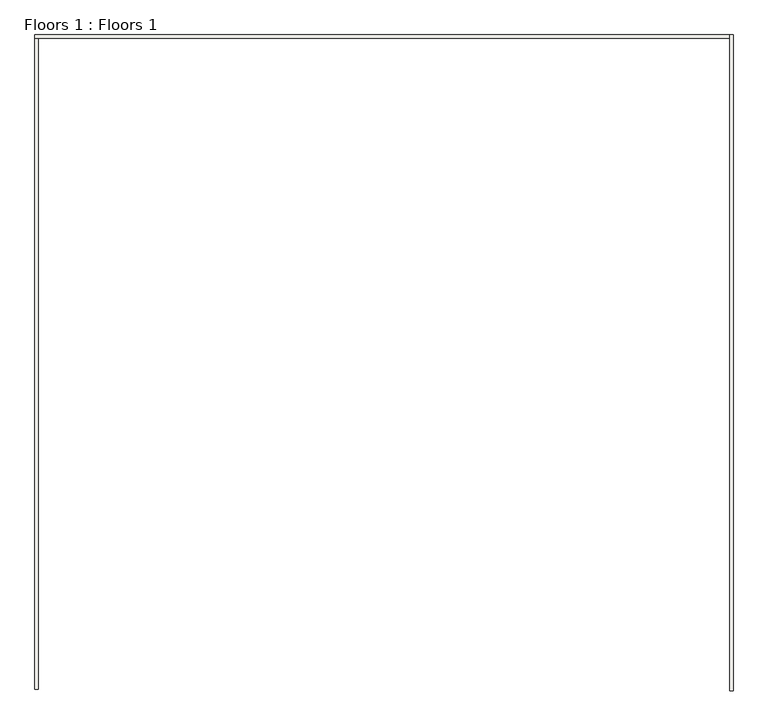
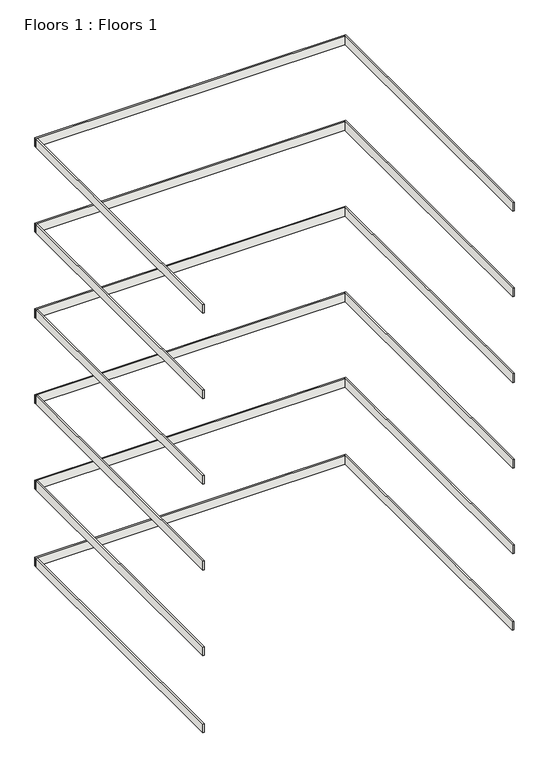
"""IFC4 building model written with IfcOpenShell, lengths in millimetres: slab geometry, Floors 1 : Floors 1."""

from ifc_helpers import new_model, si_unit, frame, origin, origin_with_axes, place, context, project, spatial, polyline, outline, extrude, source, transform, mapped, element, save


def floors_1_floors_1_bc35289f(model_context):
    return source(origin(), model_context, "Body", "SweptSolid", [
        extrude(outline(polyline([(3889.1430349, 10255.9055142), (3889.1430349, 426.1055142), (3838.3430349, 426.1055142), (3838.3430349, 10255.9055142), (3889.1430349, 10255.9055142)])), frame((0.0, 0.0, 14936.2060177), z_axis=(0.0, 0.0, 1.0), x_axis=(1.0, 0.0, 0.0)), (0.0, 0.0, 1.0), 303.7939823),
        extrude(outline(polyline([(3889.1430349, 10255.9055142), (3889.1430349, 426.1055142), (3838.3430349, 426.1055142), (3838.3430349, 10255.9055142), (3889.1430349, 10255.9055142)])), frame((0.0, 0.0, 11887.2), z_axis=(0.0, 0.0, 1.0), x_axis=(1.0, 0.0, 0.0)), (0.0, 0.0, 1.0), 304.8),
        extrude(outline(polyline([(3889.1430349, 10255.9055142), (3889.1430349, 426.1055142), (3838.3430349, 426.1055142), (3838.3430349, 10255.9055142), (3889.1430349, 10255.9055142)])), frame((0.0, 0.0, 8839.6684815), z_axis=(0.0, 0.0, 1.0), x_axis=(1.0, 0.0, 0.0)), (0.0, 0.0, 1.0), 304.3315185),
        extrude(outline(polyline([(3889.1430349, 10255.9055142), (3889.1430349, 426.1055142), (3838.3430349, 426.1055142), (3838.3430349, 10255.9055142), (3889.1430349, 10255.9055142)])), frame((0.0, 0.0, 5791.2), z_axis=(0.0, 0.0, 1.0), x_axis=(1.0, 0.0, 0.0)), (0.0, 0.0, 1.0), 304.8),
        extrude(outline(polyline([(3889.1430349, 10255.9055142), (3889.1430349, 426.1055142), (3838.3430349, 426.1055142), (3838.3430349, 10255.9055142), (3889.1430349, 10255.9055142)])), frame((0.0, 0.0, 2743.2), z_axis=(0.0, 0.0, 1.0), x_axis=(1.0, 0.0, 0.0)), (0.0, 0.0, 1.0), 304.8),
        extrude(outline(polyline([(3889.1430349, 10255.9055142), (3889.1430349, 451.5055142), (3838.3430349, 451.5055142), (3838.3430349, 10255.9055142), (3889.1430349, 10255.9055142)])), origin_with_axes(), (0.0, 0.0, 1.0), 304.8),
        extrude(outline(polyline([(-6575.6569651, 10255.9055142), (3838.3430349, 10255.9055142), (3838.3430349, 10205.1055142), (-6575.6569651, 10205.1055142), (-6575.6569651, 10255.9055142)])), frame((0.0, 0.0, 14935.2), z_axis=(0.0, 0.0, 1.0), x_axis=(1.0, 0.0, 0.0)), (0.0, 0.0, 1.0), 304.8),
        extrude(outline(polyline([(-6575.6569651, 10255.9055142), (3838.3430349, 10255.9055142), (3838.3430349, 10205.1055142), (-6575.6569651, 10205.1055142), (-6575.6569651, 10255.9055142)])), frame((0.0, 0.0, 11887.2), z_axis=(0.0, 0.0, 1.0), x_axis=(1.0, 0.0, 0.0)), (0.0, 0.0, 1.0), 304.8),
        extrude(outline(polyline([(-6575.6569651, 10255.9055142), (3838.3430349, 10255.9055142), (3838.3430349, 10205.1055142), (-6575.6569651, 10205.1055142), (-6575.6569651, 10255.9055142)])), frame((0.0, 0.0, 8839.2), z_axis=(0.0, 0.0, 1.0), x_axis=(1.0, 0.0, 0.0)), (0.0, 0.0, 1.0), 304.8),
        extrude(outline(polyline([(-6575.6569651, 10255.9055142), (3838.3430349, 10255.9055142), (3838.3430349, 10205.1055142), (-6575.6569651, 10205.1055142), (-6575.6569651, 10255.9055142)])), frame((0.0, 0.0, 5791.2), z_axis=(0.0, 0.0, 1.0), x_axis=(1.0, 0.0, 0.0)), (0.0, 0.0, 1.0), 304.8),
        extrude(outline(polyline([(-6575.6569651, 10255.9055142), (3838.3430349, 10255.9055142), (3838.3430349, 10205.1055142), (-6575.6569651, 10205.1055142), (-6575.6569651, 10255.9055142)])), frame((0.0, 0.0, 2743.2), z_axis=(0.0, 0.0, 1.0), x_axis=(1.0, 0.0, 0.0)), (0.0, 0.0, 1.0), 304.8),
        extrude(outline(polyline([(-6575.6569651, 10255.9055142), (3838.3430349, 10255.9055142), (3838.3430349, 10205.1055142), (-6575.6569651, 10205.1055142), (-6575.6569651, 10255.9055142)])), origin_with_axes(), (0.0, 0.0, 1.0), 304.8),
        extrude(outline(polyline([(-6575.6569651, 451.5055142), (-6575.6569651, 10205.1055142), (-6524.8569651, 10205.1055142), (-6524.8569651, 451.5055142), (-6575.6569651, 451.5055142)])), frame((0.0, 0.0, 14935.2), z_axis=(0.0, 0.0, 1.0), x_axis=(1.0, 0.0, 0.0)), (0.0, 0.0, 1.0), 304.8),
        extrude(outline(polyline([(-6575.6569651, 451.5055142), (-6575.6569651, 10205.1055142), (-6524.8569651, 10205.1055142), (-6524.8569651, 451.5055142), (-6575.6569651, 451.5055142)])), frame((0.0, 0.0, 11887.2), z_axis=(0.0, 0.0, 1.0), x_axis=(1.0, 0.0, 0.0)), (0.0, 0.0, 1.0), 304.8),
        extrude(outline(polyline([(-6575.6569651, 451.5055142), (-6575.6569651, 10205.1055142), (-6524.8569651, 10205.1055142), (-6524.8569651, 451.5055142), (-6575.6569651, 451.5055142)])), frame((0.0, 0.0, 8839.2), z_axis=(0.0, 0.0, 1.0), x_axis=(1.0, 0.0, 0.0)), (0.0, 0.0, 1.0), 304.8),
        extrude(outline(polyline([(-6575.6569651, 451.5055142), (-6575.6569651, 10205.1055142), (-6524.8569651, 10205.1055142), (-6524.8569651, 451.5055142), (-6575.6569651, 451.5055142)])), frame((0.0, 0.0, 5791.2), z_axis=(0.0, 0.0, 1.0), x_axis=(1.0, 0.0, 0.0)), (0.0, 0.0, 1.0), 304.8),
        extrude(outline(polyline([(-6575.6569651, 451.5055142), (-6575.6569651, 10205.1055142), (-6524.8569651, 10205.1055142), (-6524.8569651, 451.5055142), (-6575.6569651, 451.5055142)])), frame((0.0, 0.0, 2743.2), z_axis=(0.0, 0.0, 1.0), x_axis=(1.0, 0.0, 0.0)), (0.0, 0.0, 1.0), 304.8),
        extrude(outline(polyline([(-6575.6569651, 451.5055142), (-6575.6569651, 10205.1055142), (-6524.8569651, 10205.1055142), (-6524.8569651, 451.5055142), (-6575.6569651, 451.5055142)])), origin_with_axes(), (0.0, 0.0, 1.0), 304.8),
    ])


if __name__ == "__main__":
    model = new_model("IFC4")
    model_context = context("Model", 3, world=origin())
    ifc_project = project(units=[si_unit("LENGTHUNIT", "METRE", prefix="MILLI")], contexts=[model_context])
    site = spatial("IfcSite", under=ifc_project)
    building = spatial("IfcBuilding", under=site)
    placement = place(None, origin())
    floors_1_floors_1_shape = floors_1_floors_1_bc35289f(model_context)
    element("IfcSlab", 1, ObjectType="Floors 1 : Floors 1", at=placement, inside=building, context=model_context, shape_type="MappedRepresentation", body=[
        mapped(floors_1_floors_1_shape, transform((0.0, 0.0, 0.0), x_axis=(1.0, 0.0, 0.0), y_axis=(0.0, 1.0, 0.0), z_axis=(0.0, 0.0, 1.0))),
    ])
    save(model, "model.ifc")

# Revit data of these elements
# Element 1 (IfcSlab, "Floors 1 : Floors 1")
#   Materials on its faces: "1 wall brown", "Default Floor"
# Materials
#   "1 wall brown": class "Generic", colour RGB 61 46 37, transparency 0, Cost = 0
#   "Default Floor": colour RGB 128 128 128, transparency 0, Cost = 0
